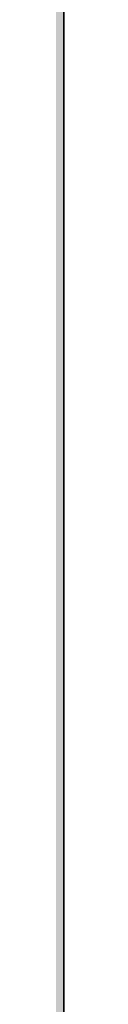
# Model space of a CAD drawing. Units: inches. Extents: x 2083 to 3317, y 1141 to 2115.
# Tile 197 of 256: x 3126.9598 to 3126.9598, y 1263.3548 to 1263.6134. Entities that reach past the tile are written whole.
import ezdxf

# ---------------------------------------------------------------- set-up
doc = ezdxf.new("R2010")
doc.units = ezdxf.units.IN
doc.layers.add('A-ANNO-DIMS', color=2, linetype='Continuous', lineweight=18)
doc.layers.add('A-WALL', color=7, linetype='Continuous', lineweight=35)
doc.layers.add('A-WALL-PATT', color=251, linetype='Continuous', lineweight=13, true_color=0x636466)
doc.styles.get("Standard").update_dxf_attribs({"font": 'arial.ttf'})
doc.dimstyles.new('ISO-25', dxfattribs={"dimtxt": 12, "dimasz": 12, "dimexe": 1.25, "dimexo": 0.625, "dimtad": 1, "dimlunit": 3, "dimtxsty": 'Standard', "dimcen": 2.5, "dimadec": 0, "dimazin": 0, "dimtfac": 1, "dimtmove": 0, "dimatfit": 3, "dimfxl": 1, "dimarcsym": 0})

# ---------------------------------------------------------------- blocks, each defined once
blk = doc.blocks.new('*D9')
at = {"layer": 'A-ANNO-DIMS', "color": 0, "lineweight": -2, "transparency": 16777216}
for p, q in [((3127.58478, 1486.76136), (3190.40309, 1486.76136)), ((3189.15309, 1474.76136), (3189.15309, 1275.26136)), ((3127.58478, 1263.26136), (3190.40309, 1263.26136))]:
    blk.add_line(p, q, dxfattribs=at)
at = {"layer": 'A-ANNO-DIMS', "color": 0, "transparency": 16777216}
for points in [[(3187.15309, 1474.76136), (3191.15309, 1474.76136), (3189.15309, 1486.76136)], [(3187.15309, 1275.26136), (3191.15309, 1275.26136), (3189.15309, 1263.26136)]]:
    blk.add_solid(points, dxfattribs=at)
at = {"layer": 'Defpoints', "color": 0, "transparency": 16777216}
for p in [(3126.95978, 1486.76136), (3126.95978, 1263.26136), (3189.15309, 1263.26136)]:
    blk.add_point(p, dxfattribs=at)
at = {"layer": 'A-ANNO-DIMS', "color": 0, "transparency": 16777216, "insert": (3182.40121, 1375.01136), "char_height": 12, "attachment_point": 5, "rotation": 90}
blk.add_mtext('18\'-7.5"', dxfattribs=at)
blk = doc.blocks.new('*D26')
at = {"layer": 'A-ANNO-DIMS', "color": 0, "lineweight": -2, "transparency": 16777216}
for p, q in [((3088.98584, 1274.91509), (3088.98584, 1270.95196)), ((3111.24004, 1274.91509), (3111.24004, 1270.95196)), ((3076.98584, 1272.20196), (2840.26245, 1272.20196)), ((3111.24004, 1272.20196), (3088.98584, 1272.20196)), ((3123.24004, 1272.20196), (3135.24004, 1272.20196))]:
    blk.add_line(p, q, dxfattribs=at)
at = {"layer": 'A-ANNO-DIMS', "color": 0, "transparency": 16777216}
for points in [[(3076.98584, 1274.20196), (3076.98584, 1270.20196), (3088.98584, 1272.20196)], [(3123.24004, 1274.20196), (3123.24004, 1270.20196), (3111.24004, 1272.20196)]]:
    blk.add_solid(points, dxfattribs=at)
at = {"layer": 'Defpoints', "color": 0, "transparency": 16777216}
for p in [(3088.98584, 1275.54009), (3111.24004, 1275.54009), (3088.98584, 1272.20196)]:
    blk.add_point(p, dxfattribs=at)
at = {"layer": 'A-ANNO-DIMS', "color": 0, "transparency": 16777216, "insert": (2952.62415, 1279.0316), "char_height": 12, "attachment_point": 5}
blk.add_mtext('NIGHTSTAND 1\'-10 1/2" TYP.', dxfattribs=at)
blk = doc.blocks.new('*D27')
at = {"layer": 'A-ANNO-DIMS', "color": 0, "lineweight": -2, "transparency": 16777216}
for p, q in [((3114.57817, 1309.79428), (3114.57817, 1321.79428)), ((3111.86504, 1297.79428), (3115.82817, 1297.79428)), ((3114.57817, 1297.79428), (3114.57817, 1275.54009)), ((3111.86504, 1275.54009), (3115.82817, 1275.54009)), ((3114.57817, 1263.54009), (3114.57817, 1140.98859))]:
    blk.add_line(p, q, dxfattribs=at)
at = {"layer": 'A-ANNO-DIMS', "color": 0, "transparency": 16777216}
for points in [[(3112.57817, 1309.79428), (3116.57817, 1309.79428), (3114.57817, 1297.79428)], [(3112.57817, 1263.54009), (3116.57817, 1263.54009), (3114.57817, 1275.54009)]]:
    blk.add_solid(points, dxfattribs=at)
at = {"layer": 'Defpoints', "color": 0, "transparency": 16777216}
for p in [(3111.24004, 1297.79428), (3111.24004, 1275.54009), (3114.57817, 1275.54009)]:
    blk.add_point(p, dxfattribs=at)
at = {"layer": 'A-ANNO-DIMS', "color": 0, "transparency": 16777216, "insert": (3107.74853, 1196.26434), "char_height": 12, "attachment_point": 5, "rotation": 90}
blk.add_mtext('1\'-10 1/2" TYP.', dxfattribs=at)

msp = doc.modelspace()

# ---------------------------------------------------------------- hatches: boundary and pattern name
at = {"layer": 'A-WALL-PATT'}
h = msp.add_hatch(color=256, dxfattribs=at)
h.dxf.hatch_style = 1
h.paths.add_polyline_path([(3126.95978, 2020.76136), (2748.95978, 2020.76136), (2604.95978, 2020.76136), (2226.95978, 2020.76136), (2226.95978, 1702.76136), (2466.95978, 1702.76136), (2466.95978, 1582.76136), (2418.95978, 1582.76136), (2418.95978, 1477.76136), (2226.95978, 1477.76136), (2226.95978, 1263.26136), (2544.95978, 1263.26136), (2544.95978, 1411.76136), (2604.95978, 1411.76136), (2685.95978, 1411.76136), (2685.95978, 1420.76136), (2604.95978, 1420.76136), (2604.95978, 1573.76136), (2604.95978, 1702.76136), (2604.95978, 2011.76136), (2748.95978, 2011.76136), (2748.95978, 1702.76136), (2862.95978, 1702.76136), (2862.95978, 1621.76136), (2871.95978, 1621.76136), (2871.95978, 1702.76136), (2883.95978, 1702.76136), (2883.95978, 1706.93946, -0.026459), (2883.95978, 1711.76136), (2757.95978, 1711.76136), (2757.95978, 1807.76136), (2787.95978, 1807.76136), (2787.95978, 1812.26136), (2757.95978, 1812.26136), (2757.95978, 2011.76136), (2877.95978, 2011.76136), (2877.95978, 1812.26136), (2847.95978, 1812.26136), (2847.95978, 1807.76136), (2889.83574, 1807.76136), (2889.83574, 1812.26136), (2882.45978, 1812.26136), (2882.45978, 2011.76136), (3117.95978, 2011.76136), (3117.95978, 1812.26136), (2937.83574, 1812.26136), (2937.83574, 1807.76136), (2995.70978, 1807.76136), (2995.70978, 1796.11767), (3000.20978, 1796.11767), (3000.20978, 1807.76136), (3117.95978, 1807.76136), (3117.95978, 1711.76136), (3000.20978, 1711.76136), (3000.20978, 1760.11767), (2998.5727, 1760.11767, -0.020711), (2995.70978, 1760.11767), (2995.70978, 1711.76136), (2931.95978, 1711.76136), (2931.95978, 1702.76136), (3126.95978, 1702.76136)])
h.paths.add_polyline_path([(2471.45978, 2011.76136), (2471.45978, 1810.01136), (2462.71694, 1810.01136), (2462.71694, 1805.51136), (2505.95978, 1805.51136), (2505.95978, 1810.01136), (2475.95978, 1810.01136), (2475.95978, 2011.76136), (2595.95978, 2011.76136), (2595.95978, 1810.01136), (2565.95978, 1810.01136), (2565.95978, 1805.51136), (2595.95978, 1805.51136), (2595.95978, 1711.76136), (2235.95978, 1711.76136), (2235.95978, 1805.51136), (2353.70978, 1805.51136), (2353.70978, 1796.05416), (2358.20978, 1796.05416), (2358.20978, 1805.51136), (2414.71694, 1805.51136), (2414.71694, 1810.01136), (2235.95978, 1810.01136), (2235.95978, 2011.76136)], flags=16)
h.paths.add_polyline_path([(2270.20473, 1994.61001), (2270.20473, 1970.61001), (2246.20473, 1970.61001), (2246.20473, 1994.61001)], flags=0)
edge = h.paths.add_edge_path(flags=0)
edge.add_ellipse((2332.02739, 1899.79818), major_axis=(-3.04299, 3.04299), ratio=0.1682525, start_angle=-161.33217, end_angle=-156.30711, ccw=False)
edge.add_ellipse((2333.08204, 1898.74353), major_axis=(-1.05465, 1.05465), ratio=0.4535321, start_angle=-123.37102, end_angle=-94.15911)
edge = h.paths.add_edge_path(flags=0)
edge.add_ellipse((2332.02739, 1968.87629), major_axis=(3.04299, 3.04299), ratio=0.1682525, start_angle=18.66783, end_angle=23.69289)
edge.add_spline(control_points=[(2332.9256, 1970.6911), (2332.22677, 1970.3361), (2330.89371, 1969.65891), (2328.41308, 1970.93214), (2327.20393, 1967.74871), (2324.7096, 1969.95559), (2322.53282, 1967.01235), (2320.01285, 1971.29581), (2317.68031, 1968.15784), (2316.04053, 1967.10205), (2315.4269, 1966.8096)], knot_values=[0, 0, 0, 0, 2.267059, 4.324559, 6.685584, 8.878641, 11.121502, 14.300359, 17.755284, 19.732645, 19.732645, 19.732645, 19.732645], degree=3, periodic=0)
edge.add_ellipse((2332.02739, 1968.87629), major_axis=(3.04299, 3.04299), ratio=0.1682525, start_angle=18.66783, end_angle=23.69289, ccw=False)
edge.add_ellipse((2333.08204, 1969.93094), major_axis=(1.05465, 1.05465), ratio=0.4535321, start_angle=56.62898, end_angle=85.84089, ccw=False)
edge = h.paths.add_edge_path(flags=0)
edge.add_spline(control_points=[(2296.42829, 1967.98791), (2293.6278, 1965.33631), (2287.70362, 1959.72709), (2299.74386, 1949.9957), (2294.53259, 1935.66853), (2290.57323, 1920.60351), (2293.39412, 1909.97369), (2296.18541, 1904.96654)], knot_values=[0.099185, 0.099185, 0.099185, 0.099185, 0.345301, 0.619822, 0.982653, 1.386093, 1.810555, 1.810555, 1.810555, 1.810555], degree=3, periodic=0)
edge.add_spline(control_points=[(2296.18541, 1904.96654), (2297.38358, 1902.6193), (2298.00097, 1901.94931), (2298.55297, 1901.46815)], knot_values=[0.006246, 0.006246, 0.006246, 0.006246, 0.055476, 0.055476, 0.055476, 0.055476], degree=3, periodic=0)
edge.add_spline(control_points=[(2298.55297, 1901.46815), (2297.25861, 1900.92322), (2295.22529, 1900.23213), (2293.06023, 1900.61421), (2292.10142, 1900.78841), (2292.08958, 1900.79057)], knot_values=[0.312835, 0.312835, 0.312835, 0.312835, 0.40178, 0.474987, 0.475903, 0.475903, 0.475903, 0.475903], degree=3, periodic=0)
edge.add_arc((2292.79365, 1904.66411), 3.93701, 215.4209, 259.69818, ccw=False)
edge.add_spline(control_points=[(2289.58531, 1902.3823), (2289.47665, 1902.53509), (2289.36848, 1902.68804), (2289.26086, 1902.84117)], knot_values=[0.102872, 0.102872, 0.102872, 0.102872, 0.116896, 0.116896, 0.116896, 0.116896], degree=3, periodic=0)
edge.add_spline(control_points=[(2289.26086, 1902.84117), (2288.6866, 1902.55019), (2287.64005, 1902.0199), (2285.88134, 1901.87395), (2283.85297, 1901.50435), (2281.71999, 1899.71054), (2278.46699, 1899.49294), (2276.15714, 1901.8832), (2272.25895, 1899.80407), (2267.77761, 1901.84318), (2262.24388, 1900.18403), (2257.41493, 1901.78206), (2254.31837, 1900.72612), (2253.17828, 1900.33734)], knot_values=[0, 0, 0, 0, 1.907977, 3.477176, 5.261074, 7.972851, 11.680248, 13.717921, 16.939592, 22.789562, 27.502503, 33.595215, 37.145618, 37.145618, 37.145618, 37.145618], degree=3, periodic=0)
edge.add_line((2253.17828, 1900.33734), (2250.24424, 1902.84117))
edge.add_line((2250.24424, 1902.84117), (2250.24424, 1965.8333))
edge.add_line((2250.24424, 1965.8333), (2253.17828, 1968.33712))
edge.add_spline(control_points=[(2253.17828, 1968.33712), (2254.31837, 1967.94835), (2257.41493, 1966.89241), (2262.24388, 1968.49043), (2267.77761, 1966.83128), (2271.52673, 1968.53722), (2273.87591, 1967.82829), (2274.2067, 1967.72764)], knot_values=[0, 0, 0, 0, 0.09018, 0.244935, 0.364644, 0.513233, 0.537855, 0.537855, 0.537855, 0.537855], degree=3, periodic=0)
edge.add_arc((2274.35289, 1963.79335), 3.93701, 72.05113, 92.12795, ccw=False)
edge.add_arc((2281.29693, 1985.23), 18.5963, 252.051134, 288.565722)
edge.add_arc((2292.31672, 1956.02888), 12.64608, 71.026788, 113.778218, ccw=False)
edge = h.paths.add_edge_path(flags=0)
edge.add_spline(control_points=[(2274.89941, 1951.85619), (2275.06616, 1951.61659), (2275.23269, 1951.37659), (2275.39799, 1951.13585)], knot_values=[1.409916, 1.409916, 1.409916, 1.409916, 1.43159, 1.43159, 1.43159, 1.43159], degree=3, periodic=0)
edge.add_spline(control_points=[(2275.39799, 1951.13585), (2275.79211, 1950.56189), (2276.17923, 1949.98377), (2276.54555, 1949.3971)], knot_values=[1.358238, 1.358238, 1.358238, 1.358238, 1.409916, 1.409916, 1.409916, 1.409916], degree=3, periodic=0)
edge.add_line((2276.54555, 1949.3971), (2277.43729, 1947.86218))
edge.add_spline(control_points=[(2277.43729, 1947.86218), (2276.30383, 1945.67311), (2274.6397, 1942.42688), (2274.63161, 1938.0939), (2272.79912, 1930.85155), (2274.35643, 1943.89705), (2275.94768, 1947.92336), (2276.54555, 1949.3971)], knot_values=[0.005632, 0.005632, 0.005632, 0.005632, 0.186014, 0.266002, 0.357087, 0.59639, 0.739732, 0.739732, 0.739732, 0.739732], degree=3, periodic=0)
edge.add_spline(control_points=[(2276.54555, 1949.3971), (2276.17923, 1949.98377), (2275.79211, 1950.56189), (2275.39799, 1951.13585)], knot_values=[1.358238, 1.358238, 1.358238, 1.358238, 1.409916, 1.409916, 1.409916, 1.409916], degree=3, periodic=0)
edge.add_spline(control_points=[(2275.39799, 1951.13585), (2274.9425, 1950.08045), (2274.20776, 1948.02527), (2273.9346, 1944.85148), (2272.46853, 1937.62749), (2273.46622, 1945.69647), (2274.70062, 1951.05947), (2274.89941, 1951.85619)], knot_values=[0.104364, 0.104364, 0.104364, 0.104364, 0.189636, 0.269624, 0.36071, 0.600013, 0.644622, 0.644622, 0.644622, 0.644622], degree=3, periodic=0)
h.paths.add_polyline_path([(2269.16751, 1963.12757, -0.357527), (2268.17063, 1960.97637, -0.092561), (2268.17063, 1939.43632, -0.357527), (2269.16751, 1937.28512, -0.357527), (2267.01631, 1938.282, -0.164785), (2254.68558, 1938.282, -0.357527), (2252.53438, 1937.28512, -0.357527), (2253.53126, 1939.43632, -0.092561), (2253.53126, 1960.97637, -0.357527), (2252.53438, 1963.12757, -0.357527), (2254.68558, 1962.13069, -0.164785), (2267.01631, 1962.13069, -0.357527)], flags=0)
h.paths.add_polyline_path([(2248.87407, 1967.8018), (2248.87407, 1957.02771), (2249.45778, 1957.02771), (2249.45778, 1911.64676), (2248.87407, 1911.64676), (2248.87407, 1900.87267), (2246.51186, 1900.87267, 0.197327), (2244.14966, 1902.45687), (2244.14966, 1966.21759, 0.197327), (2246.51186, 1967.8018)], flags=0)
h.paths.add_polyline_path([(2269.16751, 1931.38934, -0.357527), (2268.17063, 1929.23814, -0.092561), (2268.17063, 1907.6981, -0.357527), (2269.16751, 1905.54689, -0.357527), (2267.01631, 1906.54377, -0.164785), (2254.68558, 1906.54377, -0.357527), (2252.53438, 1905.54689, -0.357527), (2253.53126, 1907.6981, -0.092561), (2253.53126, 1929.23814, -0.357527), (2252.53438, 1931.38934, -0.357527), (2254.68558, 1930.39246, -0.164785), (2267.01631, 1930.39246, -0.357527)], flags=0)
edge = h.paths.add_edge_path(flags=0)
edge.add_spline(control_points=[(2276.19686, 1906.7237), (2276.16814, 1909.02893), (2276.11405, 1913.37185), (2270.59842, 1924.92498), (2273.90517, 1919.01278), (2275.92171, 1916.26206), (2275.47457, 1912.40215), (2277.25787, 1910.38062), (2276.69604, 1908.22504), (2276.64622, 1906.81302), (2276.61782, 1906.00841)], knot_values=[0, 0, 0, 0, 8.61026, 16.221274, 18.843057, 23.804898, 27.440828, 29.356102, 31.203478, 33.650687, 33.650687, 33.650687, 33.650687], degree=3, periodic=0)
edge.add_spline(control_points=[(2276.61782, 1906.00841), (2276.62331, 1905.62414), (2276.49774, 1904.62866), (2275.44178, 1903.85473), (2274.93731, 1903.08045), (2274.85908, 1902.84117)], knot_values=[0.156488, 0.156488, 0.156488, 0.156488, 0.184398, 0.231376, 0.250598, 0.250598, 0.250598, 0.250598], degree=3, periodic=0)
edge.add_line((2274.85908, 1902.84117), (2276.50598, 1902.84117))
edge.add_spline(control_points=[(2276.50598, 1902.84117), (2276.78831, 1903.08494), (2277.66507, 1904.1252), (2278.24954, 1904.34074), (2277.65387, 1908.52739), (2278.15567, 1906.22781), (2278.10046, 1905.28595), (2278.84667, 1904.06901), (2277.85679, 1903.41495), (2277.87419, 1902.99105), (2277.90356, 1902.84117)], knot_values=[0.059574, 0.059574, 0.059574, 0.059574, 0.080753, 0.103741, 0.16972, 0.176036, 0.207137, 0.240474, 0.262341, 0.27366, 0.27366, 0.27366, 0.27366], degree=3, periodic=0)
edge.add_line((2277.90356, 1902.84117), (2280.02983, 1902.84117))
edge.add_spline(control_points=[(2280.02983, 1902.84117), (2279.88822, 1903.0884), (2279.49926, 1903.98155), (2280.15228, 1905.93935), (2278.10362, 1909.65776), (2279.76239, 1907.18529), (2280.3279, 1904.87486), (2280.48511, 1903.48959), (2281.46327, 1903.24943), (2281.75834, 1902.9365), (2281.83404, 1902.84117)], knot_values=[0.013856, 0.013856, 0.013856, 0.013856, 0.034874, 0.088867, 0.107879, 0.126738, 0.158714, 0.193757, 0.217487, 0.226722, 0.226722, 0.226722, 0.226722], degree=3, periodic=0)
edge.add_spline(control_points=[(2281.83404, 1902.84117), (2281.78753, 1902.8267), (2281.64702, 1902.78299), (2281.39553, 1902.85949), (2281.08808, 1902.98524), (2280.72068, 1903.0609), (2280.33345, 1903.02573), (2280.12477, 1902.89888), (2280.02983, 1902.84117)], knot_values=[0, 0, 0, 0, 0.14413, 0.435517, 0.749276, 1.153046, 1.548371, 1.878348, 1.878348, 1.878348, 1.878348], degree=3, periodic=0)
edge.add_line((2280.02983, 1902.84117), (2277.90356, 1902.84117))
edge.add_spline(control_points=[(2277.90356, 1902.84117), (2277.89286, 1902.79586), (2277.8654, 1902.67964), (2277.60748, 1902.68748), (2277.27405, 1902.8007), (2276.83792, 1902.61977), (2276.58381, 1902.78926), (2276.50598, 1902.84117)], knot_values=[0, 0, 0, 0, 0.127189, 0.326199, 0.628009, 1.24357, 1.515331, 1.515331, 1.515331, 1.515331], degree=3, periodic=0)
edge.add_line((2276.50598, 1902.84117), (2274.85908, 1902.84117))
edge.add_spline(control_points=[(2274.85908, 1902.84117), (2274.81444, 1902.89859), (2274.72513, 1903.01345), (2274.49348, 1903.11897), (2274.24429, 1902.96054), (2273.93712, 1903.18494), (2273.61404, 1902.98314), (2273.40832, 1902.88304), (2273.32225, 1902.84117)], knot_values=[0, 0, 0, 0, 0.21843, 0.436957, 0.687977, 0.990379, 1.398396, 1.69185, 1.69185, 1.69185, 1.69185], degree=3, periodic=0)
edge.add_spline(control_points=[(2273.32225, 1902.84117), (2273.61674, 1903.44569), (2274.274, 1904.53825), (2276.02724, 1904.5737), (2276.20696, 1906.58364), (2276.19686, 1906.7237)], knot_values=[0.012227, 0.012227, 0.012227, 0.012227, 0.059472, 0.106218, 0.134458, 0.134458, 0.134458, 0.134458], degree=3, periodic=0)
h.paths.add_polyline_path([(2270.77605, 1897.78983), (2270.77605, 1873.78983), (2246.77605, 1873.78983), (2246.77605, 1897.78983)], flags=0)
h.paths.add_polyline_path([(2353.70978, 1760.00506), (2353.70978, 1760.05416), (2358.20978, 1760.05416, -0.033729)], flags=0)
h.paths.add_polyline_path([(2321.81912, 1737.52919), (2341.99533, 1737.52919, -0.414214), (2343.20327, 1736.32124), (2343.20327, 1721.0206, -0.414214), (2341.99533, 1719.81265), (2321.81912, 1719.81265, -0.414214), (2320.61117, 1721.0206), (2320.61117, 1736.32124, -0.414214)], flags=0)
h.paths.add_polyline_path([(2324.23501, 1736.32124), (2339.57944, 1736.32124, -0.414214), (2341.99533, 1733.90535), (2341.99533, 1725.44973, -0.414214), (2339.57944, 1723.03384), (2333.68059, 1723.03384), (2333.84532, 1722.04547, -0.870646), (2335.4254, 1721.82589, -0.767327), (2333.92269, 1721.42324), (2331.29102, 1721.42324, -0.767327), (2329.78832, 1721.82589, -0.870646), (2331.3684, 1722.04547), (2331.53313, 1723.03384), (2324.23501, 1723.03384, -0.414214), (2321.81912, 1725.44973), (2321.81912, 1733.90535, -0.414214)], flags=0)
h.paths.add_polyline_path([(2570.48379, 1928.61544), (2589.68379, 1928.61544), (2590.16883, 1928.61544), (2590.16883, 1904.9934), (2570.48379, 1904.9934)], flags=0)
h.paths.add_polyline_path([(2574.44732, 1927.26382, -1), (2572.82884, 1927.26382, -1)], flags=0)
h.paths.add_polyline_path([(2573.08987, 1926.94088), (2573.92503, 1927.77604), (2574.14774, 1927.55333), (2573.31258, 1926.71817)], flags=0)
h.paths.add_polyline_path([(2578.77906, 1919.72962, -1), (2571.59166, 1919.72962, -1)], flags=0)
h.paths.add_polyline_path([(2578.38536, 1919.72962, -1), (2571.98536, 1919.72962, -1)], flags=0)
h.paths.add_polyline_path([(2331.59576, 1729.47622, -1), (2333.61795, 1729.47622, -1)], flags=0)
h.paths.add_polyline_path([(2578.03423, 1927.26382, -1), (2576.41574, 1927.26382, -1)], flags=0)
h.paths.add_polyline_path([(2576.68885, 1927.53109), (2576.91156, 1927.7538), (2577.74673, 1926.91863), (2577.52402, 1926.69592)], flags=0)
h.paths.add_polyline_path([(2578.13906, 1909.85954, -1), (2572.23166, 1909.85954, -1)], flags=0)
h.paths.add_polyline_path([(2577.74536, 1909.85954, -1), (2572.62536, 1909.85954, -1)], flags=0)
h.paths.add_polyline_path([(2583.79772, 1927.26382, -1), (2582.17923, 1927.26382, -1)], flags=0)
h.paths.add_polyline_path([(2582.71865, 1927.7538), (2583.55381, 1926.91863), (2583.3311, 1926.69592), (2582.49594, 1927.53109)], flags=0)
h.paths.add_polyline_path([(2582.49594, 1927.53109), (2582.71865, 1927.7538), (2583.55381, 1926.91863), (2583.3311, 1926.69592)], flags=0)
h.paths.add_polyline_path([(2587.73906, 1920.52962, -1), (2581.83166, 1920.52962, -1)], flags=0)
h.paths.add_polyline_path([(2587.34536, 1920.52962, -1), (2582.22536, 1920.52962, -1)], flags=0)
h.paths.add_polyline_path([(2587.38462, 1927.26382, -1), (2585.76613, 1927.26382, -1)], flags=0)
h.paths.add_polyline_path([(2586.08199, 1926.98025), (2586.91716, 1927.81541), (2587.13987, 1927.5927), (2586.3047, 1926.75754)], flags=0)
h.paths.add_polyline_path([(2588.37906, 1910.65954, -1), (2581.19166, 1910.65954, -1)], flags=0)
h.paths.add_polyline_path([(2587.98536, 1910.65954, -1), (2581.58536, 1910.65954, -1)], flags=0)
h.paths.add_polyline_path([(2417.16773, 1729.4779), (2437.34394, 1729.4779, -0.414214), (2438.55188, 1728.26995), (2438.55188, 1712.96931, -0.414214), (2437.34394, 1711.76136), (2417.16773, 1711.76136, -0.414214), (2415.95978, 1712.96931), (2415.95978, 1728.26995, -0.414214)], flags=0)
h.paths.add_polyline_path([(2419.58362, 1728.26995), (2434.92805, 1728.26995, -0.414214), (2437.34394, 1725.85406), (2437.34394, 1717.39844, -0.414214), (2434.92805, 1714.98255), (2429.0292, 1714.98255), (2429.19393, 1713.99418, -0.870646), (2430.77401, 1713.7746, -0.767327), (2429.2713, 1713.37195), (2426.63963, 1713.37195, -0.767327), (2425.13693, 1713.7746, -0.870646), (2426.71701, 1713.99418), (2426.88174, 1714.98255), (2419.58362, 1714.98255, -0.414214), (2417.16773, 1717.39844), (2417.16773, 1725.85406, -0.414214)], flags=0)
h.paths.add_polyline_path([(2419.58362, 1728.26995), (2434.92805, 1728.26995, -0.414214), (2437.34394, 1725.85406), (2437.34394, 1717.39844, -0.414214), (2434.92805, 1714.98255), (2429.0292, 1714.98255), (2428.35812, 1719.00903), (2427.55282, 1719.00903), (2426.88174, 1714.98255), (2419.58362, 1714.98255, -0.414214), (2417.16773, 1717.39844), (2417.16773, 1725.85406, -0.414214)], flags=0)
h.paths.add_polyline_path([(2426.94437, 1721.42492, -1), (2428.96656, 1721.42492, -1)], flags=0)
h.paths.add_polyline_path([(2475.95978, 1702.76136), (2595.95978, 1702.76136), (2595.95978, 1582.76136), (2475.95978, 1582.76136)], flags=16)
h.paths.add_polyline_path([(2427.95978, 1573.76136), (2595.95978, 1573.76136), (2595.95978, 1468.76136), (2595.95978, 1420.76136), (2384.45978, 1420.76136), (2384.45978, 1468.76136), (2427.95978, 1468.76136)], flags=16)
h.paths.add_polyline_path([(2379.95978, 1468.76136), (2379.95978, 1420.76136), (2235.95978, 1420.76136), (2235.95978, 1468.76136)], flags=16)
h.paths.add_polyline_path([(2317.816, 1466.69577), (2337.9922, 1466.69577, -0.414214), (2339.20015, 1465.48782), (2339.20015, 1450.18718, -0.414214), (2337.9922, 1448.97923), (2317.816, 1448.97923, -0.414214), (2316.60805, 1450.18718), (2316.60805, 1465.48782, -0.414214)], flags=0)
h.paths.add_polyline_path([(2320.23189, 1465.48782), (2335.57631, 1465.48782, -0.414214), (2337.9922, 1463.07193), (2337.9922, 1454.61631, -0.414214), (2335.57631, 1452.20042), (2329.67747, 1452.20042), (2329.84219, 1451.21205, -0.870646), (2331.42228, 1450.99247, -0.767327), (2329.91957, 1450.58983), (2327.2879, 1450.58983, -0.767327), (2325.7852, 1450.99247, -0.870646), (2327.36528, 1451.21205), (2327.53001, 1452.20042), (2320.23189, 1452.20042, -0.414214), (2317.816, 1454.61631), (2317.816, 1463.07193, -0.414214)], flags=0)
h.paths.add_polyline_path([(2320.23189, 1465.48782), (2335.57631, 1465.48782, -0.414214), (2337.9922, 1463.07193), (2337.9922, 1454.61631, -0.414214), (2335.57631, 1452.20042), (2329.67747, 1452.20042), (2329.00638, 1456.22691), (2328.20109, 1456.22691), (2327.53001, 1452.20042), (2320.23189, 1452.20042, -0.414214), (2317.816, 1454.61631), (2317.816, 1463.07193, -0.414214)], flags=0)
h.paths.add_polyline_path([(2327.59264, 1458.6428, -1), (2329.61483, 1458.6428, -1)], flags=0)
h.paths.add_polyline_path([(2244.41174, 1433.34045), (2241.92094, 1433.34045, -0.414214), (2240.01786, 1435.24354), (2240.01786, 1440.95281, -0.414211), (2241.92093, 1442.8559), (2244.41174, 1442.8559, -1.976472)], flags=0)
h.paths.add_polyline_path([(2245.35689, 1434.39754, -0.414214), (2245.35689, 1441.79881, -2.144098)], flags=0)
h.paths.add_polyline_path([(2535.95978, 1416.26136), (2535.95978, 1272.26136), (2235.95978, 1272.26136), (2235.95978, 1416.26136)], flags=16)
h.paths.add_polyline_path([(2260.11956, 1384.29284), (2260.11956, 1362.03865), (2237.86537, 1362.03865), (2237.86537, 1384.29284)], flags=0)
edge = h.paths.add_edge_path(flags=0)
edge.add_line((2318.25185, 1362.0933), (2318.1458, 1362.00097))
edge.add_ellipse((2317.44512, 1360.43104), major_axis=(2.82164, 2.82164), ratio=0.1682525, start_angle=18.66783, end_angle=20.94813, ccw=False)
edge.add_ellipse((2318.42305, 1361.40897), major_axis=(0.97793, 0.97793), ratio=0.4535321, start_angle=56.62898, end_angle=70.2262, ccw=False)
edge = h.paths.add_edge_path(flags=0)
edge.add_line((2319.10737, 1295.57108), (2319.01504, 1295.67713))
edge.add_ellipse((2317.44512, 1296.37781), major_axis=(-2.82164, 2.82164), ratio=0.1682525, start_angle=-161.33217, end_angle=-159.05187, ccw=False)
edge.add_ellipse((2318.42305, 1295.39988), major_axis=(-0.97793, 0.97793), ratio=0.4535321, start_angle=-123.37102, end_angle=-109.7738)
edge = h.paths.add_edge_path(flags=0)
edge.add_spline(control_points=[(2284.21035, 1301.17022), (2284.58069, 1300.44472), (2284.89119, 1299.89202), (2285.15955, 1299.46102)], knot_values=[0.039066, 0.039066, 0.039066, 0.039066, 0.055476, 0.055476, 0.055476, 0.055476], degree=3, periodic=0)
edge.add_line((2285.15955, 1299.46102), (2284.21035, 1301.17022))
edge = h.paths.add_edge_path(flags=0)
edge.add_line((2280.41246, 1297.29801), (2283.36999, 1297.03612))
edge.add_line((2283.36999, 1297.03612), (2286.40569, 1297.92631))
edge.add_spline(control_points=[(2286.40569, 1297.92631), (2285.30549, 1297.46312), (2284.34478, 1297.12915), (2283.36999, 1297.03612)], knot_values=[0.394369, 0.394369, 0.394369, 0.394369, 0.475903, 0.475903, 0.475903, 0.475903], degree=3, periodic=0)
edge.add_spline(control_points=[(2283.36999, 1297.03612), (2283.28139, 1297.02767), (2282.31629, 1296.95734), (2281.3125, 1297.13448), (2280.42344, 1297.29602), (2280.41246, 1297.29801)], knot_values=[0.312835, 0.312835, 0.312835, 0.312835, 0.320246, 0.393453, 0.394369, 0.394369, 0.394369, 0.394369], degree=3, periodic=0)
edge = h.paths.add_edge_path(flags=0)
edge.add_line((2284.43556, 1359.60729), (2280.44629, 1355.32805))
edge.add_line((2280.44629, 1355.32805), (2279.57999, 1351.01775))
edge.add_line((2279.57999, 1351.01775), (2282.41297, 1346.58043))
edge.add_spline(control_points=[(2282.41297, 1346.58043), (2283.15333, 1345.58924), (2284.2529, 1344.0289), (2284.80104, 1342.38717), (2284.93516, 1341.80554)], knot_values=[1.240098, 1.240098, 1.240098, 1.240098, 1.332892, 1.382712, 1.382712, 1.382712, 1.382712], degree=3, periodic=0)
edge.add_spline(control_points=[(2284.93516, 1341.80554), (2285.31911, 1340.1406), (2285.23303, 1338.4092), (2284.90994, 1336.65412)], knot_values=[1.097484, 1.097484, 1.097484, 1.097484, 1.240098, 1.240098, 1.240098, 1.240098], degree=3, periodic=0)
edge.add_spline(control_points=[(2284.90994, 1336.65412), (2284.58685, 1334.89904), (2284.02675, 1333.12027), (2283.46264, 1331.36058)], knot_values=[0.95487, 0.95487, 0.95487, 0.95487, 1.097484, 1.097484, 1.097484, 1.097484], degree=3, periodic=0)
edge.add_line((2283.46264, 1331.36058), (2281.89038, 1326.15336))
edge.add_line((2281.89038, 1326.15336), (2280.75626, 1321.05609))
edge.add_line((2280.75626, 1321.05609), (2280.2992, 1316.00198))
edge.add_line((2280.2992, 1316.00198), (2280.71593, 1310.95007))
edge.add_line((2280.71593, 1310.95007), (2282.02809, 1305.97214))
edge.add_line((2282.02809, 1305.97214), (2284.21035, 1301.17022))
edge.add_spline(control_points=[(2284.21035, 1301.17022), (2283.34073, 1302.73019), (2282.6119, 1304.33649), (2282.02809, 1305.97214)], knot_values=[0.099185, 0.099185, 0.099185, 0.099185, 0.241799, 0.241799, 0.241799, 0.241799], degree=3, periodic=0)
edge.add_spline(control_points=[(2282.02809, 1305.97214), (2281.44428, 1307.60778), (2281.00549, 1309.27276), (2280.71593, 1310.95007)], knot_values=[0.241799, 0.241799, 0.241799, 0.241799, 0.384413, 0.384413, 0.384413, 0.384413], degree=3, periodic=0)
edge.add_spline(control_points=[(2280.71593, 1310.95007), (2280.43324, 1312.58761), (2280.28939, 1314.27696), (2280.29889, 1315.96203), (2280.2992, 1316.00198)], knot_values=[0.384413, 0.384413, 0.384413, 0.384413, 0.523647, 0.527028, 0.527028, 0.527028, 0.527028], degree=3, periodic=0)
edge.add_spline(control_points=[(2280.2992, 1316.00198), (2280.31233, 1317.68696), (2280.47787, 1319.36793), (2280.75626, 1321.05609)], knot_values=[0.527028, 0.527028, 0.527028, 0.527028, 0.669642, 0.669642, 0.669642, 0.669642], degree=3, periodic=0)
edge.add_spline(control_points=[(2280.75626, 1321.05609), (2281.03465, 1322.74425), (2281.42588, 1324.43961), (2281.89038, 1326.15336)], knot_values=[0.669642, 0.669642, 0.669642, 0.669642, 0.812256, 0.812256, 0.812256, 0.812256], degree=3, periodic=0)
edge.add_spline(control_points=[(2281.89038, 1326.15336), (2282.26438, 1327.53325), (2282.78787, 1329.26181), (2283.35275, 1331.01778), (2283.46264, 1331.36058)], knot_values=[0.812256, 0.812256, 0.812256, 0.812256, 0.927087, 0.95487, 0.95487, 0.95487, 0.95487], degree=3, periodic=0)
edge.add_line((2283.46264, 1331.36058), (2284.90994, 1336.65412))
edge.add_line((2284.90994, 1336.65412), (2284.93516, 1341.80554))
edge.add_line((2284.93516, 1341.80554), (2282.41297, 1346.58043))
edge.add_spline(control_points=[(2282.41297, 1346.58043), (2281.27513, 1348.10379), (2280.07845, 1349.57032), (2279.57999, 1351.01775)], knot_values=[1.382712, 1.382712, 1.382712, 1.382712, 1.525326, 1.525326, 1.525326, 1.525326], degree=3, periodic=0)
edge.add_spline(control_points=[(2279.57999, 1351.01775), (2279.44328, 1351.41472), (2279.13631, 1352.85692), (2279.73519, 1354.29039), (2280.44629, 1355.32805)], knot_values=[1.525326, 1.525326, 1.525326, 1.525326, 1.564439, 1.667941, 1.667941, 1.667941, 1.667941], degree=3, periodic=0)
edge.add_spline(control_points=[(2280.44629, 1355.32805), (2281.42611, 1356.75784), (2282.93084, 1358.18256), (2284.43556, 1359.60729)], knot_values=[1.667941, 1.667941, 1.667941, 1.667941, 1.810555, 1.810555, 1.810555, 1.810555], degree=3, periodic=0)
edge.add_arc((2280.62307, 1348.51818), 11.72618, 71.026788, 113.778218)
edge.add_arc((2270.40489, 1375.59516), 17.24357, 252.051134, 288.565722, ccw=False)
edge.add_arc((2263.96597, 1355.71785), 3.65062, 72.05113, 92.12795)
edge.add_arc((2263.96597, 1355.71785), 3.65062, 92.12795, 177.98513)
edge.add_spline(control_points=[(2260.3176, 1355.8462), (2260.26042, 1354.22067), (2260.55128, 1350.18655), (2262.99934, 1346.76625), (2264.47274, 1344.64902)], knot_values=[1.43159, 1.43159, 1.43159, 1.43159, 1.564144, 1.770695, 1.770695, 1.770695, 1.770695], degree=3, periodic=0)
edge.add_line((2264.47274, 1344.64902), (2264.93559, 1343.98253))
edge.add_spline(control_points=[(2263.80104, 1340.24811), (2263.84324, 1340.51409), (2264.06724, 1341.75647), (2264.51269, 1343.00245), (2264.93505, 1343.98108)], knot_values=[0.53657, 0.53657, 0.53657, 0.53657, 0.559349, 0.644622, 0.644622, 0.644622, 0.644622], degree=3, periodic=0)
edge.add_spline(control_points=[(2264.93505, 1343.98108), (2265.11777, 1343.71497), (2265.29888, 1343.44791), (2265.47676, 1343.17936)], knot_values=[1.384077, 1.384077, 1.384077, 1.384077, 1.409916, 1.409916, 1.409916, 1.409916], degree=3, periodic=0)
edge.add_spline(control_points=[(2265.47676, 1343.17936), (2265.65464, 1342.91082), (2265.8293, 1342.64081), (2265.99913, 1342.36881)], knot_values=[1.358238, 1.358238, 1.358238, 1.358238, 1.384077, 1.384077, 1.384077, 1.384077], degree=3, periodic=0)
edge.add_line((2265.99913, 1342.36881), (2266.82601, 1340.94555))
edge.add_spline(control_points=[(2266.82601, 1340.94555), (2268.8944, 1337.08969), (2271.39817, 1325.843), (2270.51616, 1310.56856), (2275.91938, 1301.86061), (2277.78951, 1299.19945)], knot_values=[0.116896, 0.116896, 0.116896, 0.116896, 0.472987, 1.050969, 1.313793, 1.313793, 1.313793, 1.313793], degree=3, periodic=0)
edge.add_spline(control_points=[(2277.78951, 1299.19945), (2277.83941, 1299.12845), (2277.88943, 1299.0575), (2277.93957, 1298.98658)], knot_values=[0.109884, 0.109884, 0.109884, 0.109884, 0.116896, 0.116896, 0.116896, 0.116896], degree=3, periodic=0)
edge.add_line((2277.93957, 1298.98658), (2277.78885, 1299.19911))
edge.add_spline(control_points=[(2277.78885, 1299.19911), (2277.25658, 1298.92941), (2276.28635, 1298.4379), (2275.03935, 1298.33442), (2274.38333, 1298.2389), (2274.21525, 1298.20934)], knot_values=[33.12187, 33.12187, 33.12187, 33.12187, 35.029056, 36.598255, 37.144827, 37.144827, 37.144827, 37.144827], degree=3, periodic=0)
edge.add_line((2274.21525, 1298.20934), (2273.07315, 1297.89296))
edge.add_spline(control_points=[(2273.07315, 1297.89296), (2272.32294, 1297.57978), (2271.03915, 1296.51051), (2269.24839, 1296.22606), (2268.4231, 1296.37465)], knot_values=[26.532584, 26.532584, 26.532584, 26.532584, 29.198919, 31.839101, 31.839101, 31.839101, 31.839101], degree=3, periodic=0)
edge.add_line((2268.4231, 1296.37465), (2263.8785, 1297.45753))
edge.add_spline(control_points=[(2263.8785, 1297.45753), (2263.55608, 1297.35943), (2261.86031, 1296.83869), (2260.23878, 1297.28241), (2258.93345, 1297.51646)], knot_values=[15.919551, 15.919551, 15.919551, 15.919551, 16.939592, 21.226067, 21.226067, 21.226067, 21.226067], degree=3, periodic=0)
edge.add_line((2258.93345, 1297.51646), (2254.05523, 1297.32901))
edge.add_spline(control_points=[(2254.05523, 1297.32901), (2253.75553, 1297.29582), (2252.11368, 1297.16517), (2250.46187, 1297.54422), (2249.12969, 1297.66788)], knot_values=[5.306517, 5.306517, 5.306517, 5.306517, 6.276435, 10.613034, 10.613034, 10.613034, 10.613034], degree=3, periodic=0)
edge.add_line((2249.12969, 1297.66788), (2244.33165, 1296.87776))
edge.add_line((2244.33165, 1296.87776), (2241.61103, 1299.19945))
edge.add_line((2241.61103, 1299.19945), (2241.61103, 1357.6094))
edge.add_line((2241.61103, 1357.6094), (2244.33165, 1359.9311))
edge.add_line((2244.33165, 1359.9311), (2252.72882, 1359.54269))
edge.add_spline(control_points=[(2252.72882, 1359.54269), (2252.87094, 1359.54644), (2253.30574, 1359.54817), (2253.73984, 1359.51427), (2254.03174, 1359.48243)], knot_values=[0.233291, 0.233291, 0.233291, 0.233291, 0.244935, 0.268927, 0.268927, 0.268927, 0.268927], degree=3, periodic=0)
edge.add_line((2254.03174, 1359.48243), (2259.58719, 1359.41639))
edge.add_spline(control_points=[(2259.58719, 1359.41639), (2260.67707, 1359.6285), (2262.0732, 1359.897), (2263.52369, 1359.45928), (2263.83042, 1359.36595)], knot_values=[0.422516, 0.422516, 0.422516, 0.422516, 0.513233, 0.537855, 0.537855, 0.537855, 0.537855], degree=3, periodic=0)
edge.add_arc((2263.96597, 1355.71785), 3.65062, 72.05113, 92.12795, ccw=False)
edge.add_arc((2270.40489, 1375.59516), 17.24357, 252.051134, 288.565722)
edge.add_arc((2280.62307, 1348.51818), 11.72618, 71.026788, 113.778218, ccw=False)
h.paths.add_polyline_path([(2240.34053, 1359.43471), (2240.34053, 1349.44435), (2240.88178, 1349.44435), (2240.88178, 1307.3645), (2240.34053, 1307.3645), (2240.34053, 1297.37414), (2238.15016, 1297.37414, 0.197327), (2235.95978, 1298.84311), (2235.95978, 1357.96575, 0.197327), (2238.15016, 1359.43471)], flags=0)
h.paths.add_polyline_path([(2259.15779, 1355.1005, -0.357527), (2258.23342, 1353.10578, -0.092561), (2258.23342, 1333.1326, -0.357527), (2259.15779, 1331.13788, -0.357527), (2257.16307, 1332.06225, -0.164785), (2245.7293, 1332.06225, -0.357527), (2243.73458, 1331.13788, -0.357527), (2244.65895, 1333.1326, -0.092561), (2244.65895, 1353.10578, -0.357527), (2243.73458, 1355.1005, -0.357527), (2245.7293, 1354.17613, -0.164785), (2257.16307, 1354.17613, -0.357527)], flags=0)
edge = h.paths.add_edge_path(flags=0)
edge.add_line((2265.99913, 1342.36881), (2266.82601, 1340.94555))
edge.add_line((2266.82601, 1340.94555), (2265.30756, 1337.81407))
edge.add_line((2265.30756, 1337.81407), (2264.35823, 1334.65294))
edge.add_line((2264.35823, 1334.65294), (2264.26201, 1333.7997))
edge.add_spline(control_points=[(2264.26201, 1333.7997), (2264.20836, 1333.18705), (2264.16206, 1332.36553), (2264.00714, 1331.41393), (2263.96905, 1331.20183)], knot_values=[0.464444, 0.464444, 0.464444, 0.464444, 0.516691, 0.531608, 0.531608, 0.531608, 0.531608], degree=3, periodic=0)
edge.add_spline(control_points=[(2263.96905, 1331.20183), (2263.77453, 1330.11887), (2263.42437, 1328.79084), (2263.25742, 1328.53065), (2263.23403, 1328.51461)], knot_values=[0.372682, 0.372682, 0.372682, 0.372682, 0.44885, 0.464444, 0.464444, 0.464444, 0.464444], degree=3, periodic=0)
edge.add_spline(control_points=[(2263.23403, 1328.51461), (2263.09638, 1328.42023), (2263.13117, 1329.30148), (2263.27495, 1330.61575)], knot_values=[0.280919, 0.280919, 0.280919, 0.280919, 0.372682, 0.372682, 0.372682, 0.372682], degree=3, periodic=0)
edge.add_spline(control_points=[(2263.27495, 1330.61575), (2263.41874, 1331.93002), (2263.67152, 1333.67732), (2263.96985, 1335.31503)], knot_values=[0.189157, 0.189157, 0.189157, 0.189157, 0.280919, 0.280919, 0.280919, 0.280919], degree=3, periodic=0)
edge.add_spline(control_points=[(2263.96985, 1335.31503), (2264.1005, 1336.03219), (2264.41878, 1337.62191), (2264.75485, 1338.86443), (2264.94742, 1339.49112)], knot_values=[0.097394, 0.097394, 0.097394, 0.097394, 0.137578, 0.189157, 0.189157, 0.189157, 0.189157], degree=3, periodic=0)
edge.add_spline(control_points=[(2264.94742, 1339.49112), (2265.29002, 1340.60605), (2265.64424, 1341.494), (2265.99913, 1342.36881)], knot_values=[0.005632, 0.005632, 0.005632, 0.005632, 0.097394, 0.097394, 0.097394, 0.097394], degree=3, periodic=0)
h.paths.add_polyline_path([(2259.15779, 1325.67097, -0.357527), (2258.23342, 1323.67625, -0.092561), (2258.23342, 1303.70307, -0.357527), (2259.15779, 1301.70835, -0.357527), (2257.16307, 1302.63272, -0.164785), (2245.7293, 1302.63272, -0.357527), (2243.73458, 1301.70835, -0.357527), (2244.65895, 1303.70307, -0.092561), (2244.65895, 1323.67625, -0.357527), (2243.73458, 1325.67097, -0.357527), (2245.7293, 1324.74661, -0.164785), (2257.16307, 1324.74661, -0.357527)], flags=0)
edge = h.paths.add_edge_path(flags=0)
edge.add_spline(control_points=[(2261.70894, 1317.31142), (2261.67948, 1317.41758), (2261.76186, 1317.38853), (2262.49074, 1316.08987), (2262.96218, 1315.3009)], knot_values=[14.955861, 14.955861, 14.955861, 14.955861, 16.221274, 18.694826, 18.694826, 18.694826, 18.694826], degree=3, periodic=0)
edge.add_spline(control_points=[(2262.96218, 1315.3009), (2262.99044, 1315.25362), (2263.7021, 1314.06738), (2264.34898, 1313.12715), (2264.73005, 1312.16415)], knot_values=[18.694826, 18.694826, 18.694826, 18.694826, 18.843057, 22.433791, 22.433791, 22.433791, 22.433791], degree=3, periodic=0)
edge.add_spline(control_points=[(2264.73005, 1312.16415), (2264.87556, 1311.79644), (2265.17687, 1310.76981), (2265.14307, 1309.55926), (2265.24774, 1308.82419)], knot_values=[22.433791, 22.433791, 22.433791, 22.433791, 23.804898, 26.172756, 26.172756, 26.172756, 26.172756], degree=3, periodic=0)
edge.add_line((2265.24774, 1308.82419), (2265.85077, 1307.17189))
edge.add_spline(control_points=[(2265.85077, 1307.17189), (2266.06502, 1306.82168), (2266.38439, 1306.33225), (2266.4244, 1305.78055), (2266.42037, 1305.61122)], knot_values=[28.062562, 28.062562, 28.062562, 28.062562, 29.356102, 29.911721, 29.911721, 29.911721, 29.911721], degree=3, periodic=0)
edge.add_spline(control_points=[(2266.42037, 1305.61122), (2266.41612, 1305.43259), (2266.394, 1305.25), (2266.36478, 1305.06586)], knot_values=[29.911721, 29.911721, 29.911721, 29.911721, 30.497837, 30.497837, 30.497837, 30.497837], degree=3, periodic=0)
edge.add_line((2266.36478, 1305.06586), (2266.06615, 1302.1363))
edge.add_spline(control_points=[(2266.06615, 1302.1363), (2266.07124, 1301.77998), (2265.99808, 1301.19998), (2265.66327, 1300.75896), (2265.50891, 1300.58588)], knot_values=[0.156488, 0.156488, 0.156488, 0.156488, 0.184398, 0.203543, 0.203543, 0.203543, 0.203543], degree=3, periodic=0)
edge.add_line((2265.50891, 1300.58588), (2264.43534, 1299.19945))
edge.add_line((2264.43534, 1299.19945), (2265.96244, 1299.19945))
edge.add_line((2265.96244, 1299.19945), (2267.33599, 1301.17528))
edge.add_line((2267.33599, 1301.17528), (2267.31167, 1301.98624))
edge.add_spline(control_points=[(2267.31167, 1301.98624), (2267.26111, 1302.8624), (2267.16021, 1303.73713), (2267.27149, 1303.3259)], knot_values=[0.126229, 0.126229, 0.126229, 0.126229, 0.166617, 0.166617, 0.166617, 0.166617], degree=3, periodic=0)
edge.add_spline(control_points=[(2267.27149, 1303.3259), (2267.28003, 1303.2943), (2267.30979, 1303.17537), (2267.37345, 1302.88361), (2267.40612, 1302.68283), (2267.41793, 1302.60103)], knot_values=[0.166617, 0.166617, 0.166617, 0.166617, 0.16972, 0.176036, 0.180765, 0.180765, 0.180765, 0.180765], degree=3, periodic=0)
edge.add_spline(control_points=[(2267.74389, 1300.9875), (2267.68758, 1301.15094), (2267.48052, 1301.65666), (2267.48375, 1302.14479), (2267.41793, 1302.60103)], knot_values=[0.180765, 0.180765, 0.180765, 0.180765, 0.193767, 0.220139, 0.220139, 0.220139, 0.220139], degree=3, periodic=0)
edge.add_line((2267.41793, 1302.60103), (2267.74389, 1300.9875))
edge.add_spline(control_points=[(2267.74389, 1300.9875), (2267.83196, 1300.73188), (2267.93202, 1300.3099), (2267.55484, 1299.97452), (2267.42937, 1299.82921)], knot_values=[0.220139, 0.220139, 0.220139, 0.220139, 0.240474, 0.25489, 0.25489, 0.25489, 0.25489], degree=3, periodic=0)
edge.add_line((2267.42937, 1299.82921), (2267.25836, 1299.19945))
edge.add_line((2267.25836, 1299.19945), (2269.22996, 1299.19945))
edge.add_spline(control_points=[(2269.22996, 1299.19945), (2269.09865, 1299.42869), (2268.84277, 1300.01625), (2269.01157, 1300.91592), (2268.9468, 1301.66074)], knot_values=[0.013856, 0.013856, 0.013856, 0.013856, 0.034874, 0.067073, 0.067073, 0.067073, 0.067073], degree=3, periodic=0)
edge.add_line((2268.9468, 1301.66074), (2268.43158, 1303.60311))
edge.add_spline(control_points=[(2268.43158, 1303.60311), (2268.1756, 1304.19237), (2267.59621, 1305.2513), (2268.0407, 1304.62321), (2268.25139, 1304.28242)], knot_values=[0.090155, 0.090155, 0.090155, 0.090155, 0.107879, 0.120289, 0.120289, 0.120289, 0.120289], degree=3, periodic=0)
edge.add_spline(control_points=[(2268.25139, 1304.28242), (2268.36088, 1304.10533), (2269.05775, 1302.91798), (2269.38269, 1301.59042), (2269.52141, 1300.77593), (2269.57522, 1300.55578)], knot_values=[0.120289, 0.120289, 0.120289, 0.120289, 0.126738, 0.158714, 0.173506, 0.173506, 0.173506, 0.173506], degree=3, periodic=0)
edge.add_line((2269.57522, 1300.55578), (2270.6858, 1299.42126))
edge.add_spline(control_points=[(2270.6858, 1299.42126), (2270.76722, 1299.35725), (2270.83785, 1299.2814), (2270.90292, 1299.19945)], knot_values=[0.21816, 0.21816, 0.21816, 0.21816, 0.226722, 0.226722, 0.226722, 0.226722], degree=3, periodic=0)
edge.add_line((2270.9372, 1299.19291), (2270.90292, 1299.19945))
edge.add_spline(control_points=[(2270.90292, 1299.19945), (2270.85981, 1299.18603), (2270.72951, 1299.1455), (2270.49631, 1299.21644), (2270.27166, 1299.30832), (2270.12102, 1299.34796), (2270.06334, 1299.35956)], knot_values=[0.939174, 0.939174, 0.939174, 0.939174, 1.083304, 1.374691, 1.68845, 1.878348, 1.878348, 1.878348, 1.878348], degree=3, periodic=0)
edge.add_line((2270.06334, 1299.35956), (2269.22996, 1299.19945))
edge.add_line((2269.22996, 1299.19945), (2267.25836, 1299.19945))
edge.add_spline(control_points=[(2267.25836, 1299.19945), (2267.24843, 1299.15743), (2267.22297, 1299.04967), (2266.98382, 1299.05694), (2266.80921, 1299.11623), (2266.6769, 1299.10909), (2266.63653, 1299.10481)], knot_values=[0.757665, 0.757665, 0.757665, 0.757665, 0.884854, 1.083864, 1.385675, 1.515331, 1.515331, 1.515331, 1.515331], degree=3, periodic=0)
edge.add_spline(control_points=[(2266.63653, 1299.10481), (2266.48522, 1299.08879), (2266.23581, 1299.01712), (2266.03461, 1299.15132), (2265.96244, 1299.19945)], knot_values=[0, 0, 0, 0, 0.485905, 0.757665, 0.757665, 0.757665, 0.757665], degree=3, periodic=0)
edge.add_line((2265.96244, 1299.19945), (2264.43534, 1299.19945))
edge.add_line((2264.43534, 1299.19945), (2263.85844, 1299.36712))
edge.add_spline(control_points=[(2263.85844, 1299.36712), (2263.81894, 1299.37091), (2263.77953, 1299.38572), (2263.74013, 1299.4015)], knot_values=[0.845925, 0.845925, 0.845925, 0.845925, 0.978627, 0.978627, 0.978627, 0.978627], degree=3, periodic=0)
edge.add_line((2263.72179, 1299.39643), (2263.01031, 1299.19945))
edge.add_spline(control_points=[(2263.01031, 1299.19945), (2263.24579, 1299.68286), (2263.50603, 1300.12811), (2263.87349, 1300.40803)], knot_values=[0.012227, 0.012227, 0.012227, 0.012227, 0.052971, 0.052971, 0.052971, 0.052971], degree=3, periodic=0)
edge.add_spline(control_points=[(2263.87349, 1300.40803), (2263.93213, 1300.4527), (2264.08424, 1300.55298), (2264.25519, 1300.62422), (2264.35969, 1300.66475)], knot_values=[0.052971, 0.052971, 0.052971, 0.052971, 0.059472, 0.069086, 0.069086, 0.069086, 0.069086], degree=3, periodic=0)
edge.add_line((2264.35969, 1300.66475), (2265.1419, 1301.07777))
edge.add_line((2265.1419, 1301.07777), (2265.67581, 1302.79956))
edge.add_line((2265.67581, 1302.79956), (2265.5407, 1305.70407))
edge.add_line((2265.5407, 1305.70407), (2264.80307, 1309.32772))
edge.add_line((2264.80307, 1309.32772), (2263.04053, 1314.09179))
edge.add_spline(control_points=[(2263.04053, 1314.09179), (2262.38357, 1315.67144), (2261.79597, 1316.99775), (2261.70894, 1317.31142)], knot_values=[11.216896, 11.216896, 11.216896, 11.216896, 14.955861, 14.955861, 14.955861, 14.955861], degree=3, periodic=0)
h.paths.add_polyline_path([(2871.95978, 1416.26136), (2895.91005, 1416.26136), (2895.91005, 1420.76136), (2871.95978, 1420.76136), (2871.95978, 1501.76136), (2862.95978, 1501.76136), (2862.95978, 1420.76136), (2805.95978, 1420.76136), (2805.95978, 1411.76136), (2862.95978, 1411.76136), (2862.95978, 1263.26136), (3126.95978, 1263.26136), (3126.95978, 1411.76136), (3126.95978, 1486.76136), (2943.95978, 1486.76136), (2943.95978, 1477.76136), (2967.86031, 1477.76136), (2967.86031, 1420.76136), (2943.91005, 1420.76136), (2943.91005, 1416.26136), (3117.95978, 1416.26136), (3117.95978, 1420.76136), (2972.36031, 1420.76136), (2972.36031, 1477.76136), (3117.95978, 1477.76136), (3117.95978, 1420.76136), (3117.95978, 1272.26136), (2871.95978, 1272.26136)], flags=0)
h.paths.add_polyline_path([(2457.12563, 1485.94251), (2527.60265, 1485.94251), (2527.60265, 1537.6357), (2457.12563, 1537.6357)], flags=8)
h.paths.add_polyline_path([(2481.00506, 1609.9818), (2590.76582, 1609.9818), (2590.76582, 1682.00336), (2481.00506, 1682.00336)], flags=8)
h.paths.add_polyline_path([(2483.08502, 1729.12678), (2553.56205, 1729.12678), (2553.56205, 1780.81998), (2483.08502, 1780.81998)], flags=8)
h = msp.add_hatch(color=256, dxfattribs=at)
h.dxf.hatch_style = 1
h.paths.add_polyline_path([(3126.95978, 1486.76136), (2943.95978, 1486.76136), (2943.95978, 1477.76136), (2967.86031, 1477.76136), (2967.86031, 1420.76136), (2943.91005, 1420.76136), (2943.91005, 1416.26136), (3117.95978, 1416.26136), (3117.95978, 1420.76136), (2972.36031, 1420.76136), (2972.36031, 1477.76136), (3117.95978, 1477.76136), (3117.95978, 1420.76136), (3117.95978, 1272.26136), (2871.95978, 1272.26136), (2871.95978, 1416.26136), (2895.91005, 1416.26136), (2895.91005, 1420.76136), (2871.95978, 1420.76136), (2871.95978, 1501.76136), (2862.95978, 1501.76136), (2862.95978, 1420.76136), (2805.95978, 1420.76136), (2805.95978, 1411.76136), (2862.95978, 1411.76136), (2862.95978, 1263.26136), (3126.95978, 1263.26136), (3126.95978, 1411.76136)])

# ---------------------------------------------------------------- linework, layer by layer
at = {"layer": 'A-WALL'}
msp.add_line((3126.95978, 1411.76136), (3126.95978, 1263.26136), dxfattribs=at)

# ---------------------------------------------------------------- dimensions: what is measured, and where the dimension line sits
at = {"layer": 'A-ANNO-DIMS'}
dim = msp.add_linear_dim(base=(3189.15309, 1263.26136), p1=(3126.95978, 1486.76136), p2=(3126.95978, 1263.26136), angle=90, dimstyle='ISO-25', override={"dimclrd": 0, "dimclre": 0, "dimclrt": 0}, dxfattribs=at)
dim.commit()
dim.dimension.update_dxf_attribs({"geometry": '*D9', "text_midpoint": (3182.40121, 1375.01136)})
for base, p1, p2, angle, text, picture, middle in [((3114.57817, 1275.54009), (3111.24004, 1297.79428), (3111.24004, 1275.54009), 270, '<> TYP.', '*D27', (3107.74853, 1196.26434)), ((3088.98584, 1272.20196), (3111.24004, 1275.54009), (3088.98584, 1275.54009), 180, 'NIGHTSTAND <> TYP.', '*D26', (2952.62415, 1279.0316))]:
    dim = msp.add_linear_dim(base=base, p1=p1, p2=p2, angle=angle, text=text, dimstyle='ISO-25', override={"dimdec": 1, "dimlfac": 1, "dimrnd": 0, "dimzin": 1, "dimdsep": 46, "dimlunit": 4, "dimfrac": 2}, dxfattribs=at)
    dim.commit()
    dim.dimension.update_dxf_attribs({"geometry": picture, "text_midpoint": middle})

doc.saveas('drawing.dxf')
